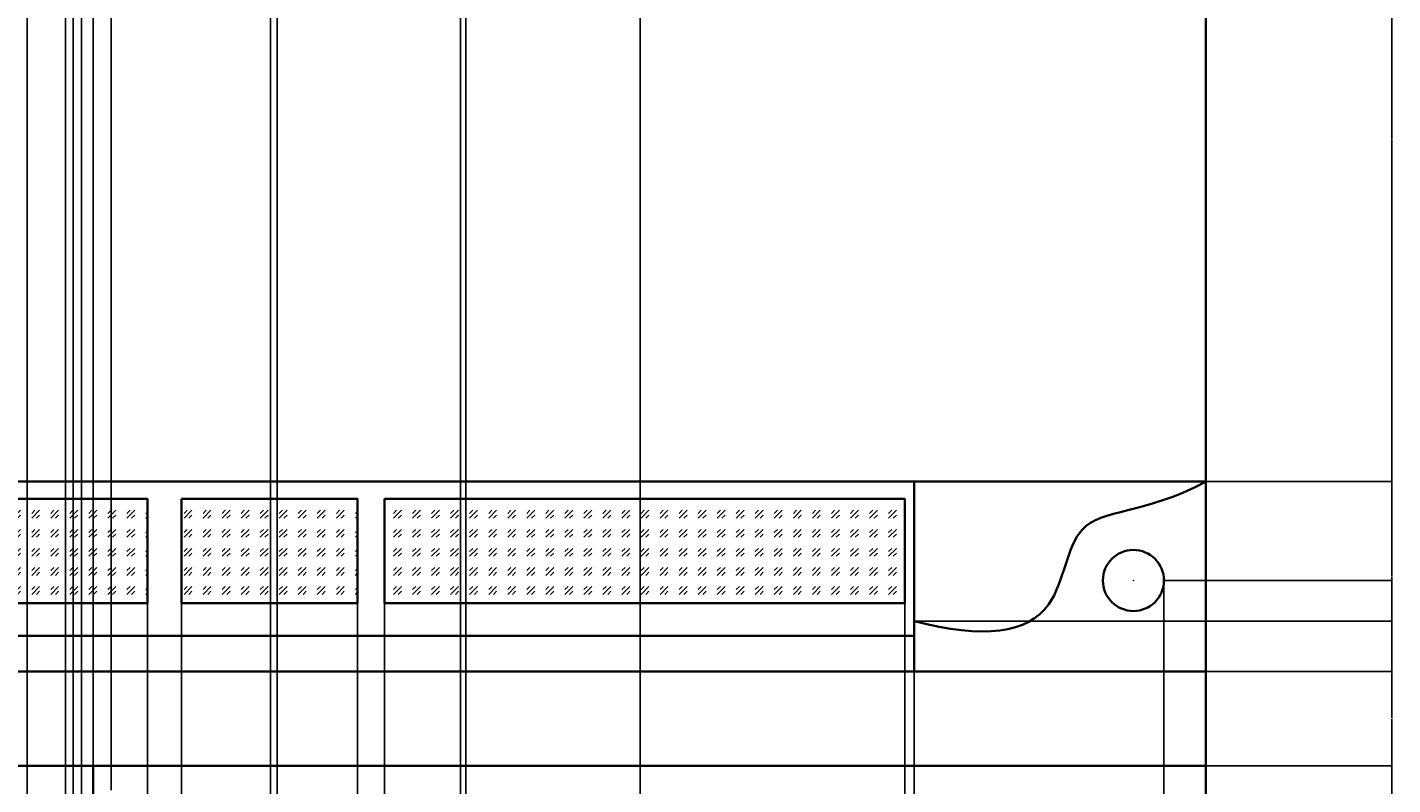
# Model space of a CAD drawing. Units: inches. Extents: x 1231 to 2151, y 481 to 2277.
# Tile 4 of 7: x 1542 to 2151, y 1035 to 1373. Entities that reach past the tile are written whole.
import ezdxf

# ---------------------------------------------------------------- set-up
doc = ezdxf.new("R2010")
doc.units = ezdxf.units.IN
doc.header["$MEASUREMENT"] = 0
for name, color, linetype, lineweight in [('A-ANNO-DIMS', 2, 'Continuous', 18), ('A-ELEV', 7, 'Continuous', 35), ('A-ELEV-PATT', 9, 'Continuous', 13)]:
    doc.layers.add(name, color=color, linetype=linetype, lineweight=lineweight)
doc.styles.get("Standard").update_dxf_attribs({"font": 'arial.ttf'})
doc.dimstyles.get("Standard").update_dxf_attribs({"dimtxt": 0.18, "dimasz": 0.18, "dimexe": 0.18, "dimexo": 0.0625, "dimgap": 0.09, "dimtad": 0, "dimtih": 1, "dimtoh": 1, "dimdec": 0, "dimzin": 0, "dimdsep": 46, "dimlunit": 3, "dimtxsty": 'Standard', "dimcen": 0.09, "dimadec": 0, "dimazin": 0, "dimtfac": 1, "dimtdec": 0, "dimtofl": 0, "dimtmove": 0, "dimatfit": 3, "dimfxl": 1, "dimtolj": 1, "dimtzin": 0, "dimarcsym": 0})

# ---------------------------------------------------------------- blocks, each defined once
blk = doc.blocks.new('*D4')
at = {"layer": 'A-ANNO-DIMS', "color": 0, "lineweight": -2, "transparency": 16777216}
for p, q in [((2067.75, 1043.69), (2150.62, 1043.69)), ((2150.44, 1043.51), (2150.44, 863.87)), ((2150.44, 683.87), (2150.44, 863.51)), ((2067.75, 683.69), (2150.62, 683.69))]:
    blk.add_line(p, q, dxfattribs=at)
at = {"layer": 'A-ANNO-DIMS', "color": 0, "transparency": 16777216}
for points in [[(2150.41, 1043.51), (2150.47, 1043.51), (2150.44, 1043.69)], [(2150.41, 683.87), (2150.47, 683.87), (2150.44, 683.69)]]:
    blk.add_solid(points, dxfattribs=at)
at = {"layer": 'Defpoints', "color": 0, "transparency": 16777216}
for p in [(2067.69, 1043.69), (2150.44, 1043.69), (2067.69, 683.69)]:
    blk.add_point(p, dxfattribs=at)
at = {"layer": 'A-ANNO-DIMS', "color": 0, "transparency": 16777216, "insert": (2150.44, 863.69), "char_height": 0.18, "attachment_point": 5}
blk.add_mtext('\\A1;360', dxfattribs=at)
blk = doc.blocks.new('*D5')
at = {"layer": 'A-ANNO-DIMS', "color": 0, "lineweight": -2, "transparency": 16777216}
for p, q in [((2067.75, 1085.71), (2150.62, 1085.71)), ((2150.44, 1085.53), (2150.44, 1064.88)), ((2150.44, 1043.87), (2150.44, 1064.52)), ((2067.75, 1043.69), (2150.62, 1043.69))]:
    blk.add_line(p, q, dxfattribs=at)
at = {"layer": 'A-ANNO-DIMS', "color": 0, "transparency": 16777216}
for points in [[(2150.41, 1085.53), (2150.47, 1085.53), (2150.44, 1085.71)], [(2150.41, 1043.87), (2150.47, 1043.87), (2150.44, 1043.69)]]:
    blk.add_solid(points, dxfattribs=at)
at = {"layer": 'Defpoints', "color": 0, "transparency": 16777216}
for p in [(2067.69, 1085.71), (2150.44, 1085.71), (2067.69, 1043.69)]:
    blk.add_point(p, dxfattribs=at)
at = {"layer": 'A-ANNO-DIMS', "color": 0, "transparency": 16777216, "insert": (2150.44, 1064.7), "char_height": 0.18, "attachment_point": 5}
blk.add_mtext('\\A1;42.02', dxfattribs=at)
blk = doc.blocks.new('*D6')
at = {"layer": 'A-ANNO-DIMS', "color": 0, "lineweight": -2, "transparency": 16777216}
for p, q in [((2067.75, 1170.34), (2150.62, 1170.34)), ((2150.44, 1170.16), (2150.44, 1128.2)), ((2150.44, 1085.89), (2150.44, 1127.84)), ((2067.75, 1085.71), (2150.62, 1085.71))]:
    blk.add_line(p, q, dxfattribs=at)
at = {"layer": 'A-ANNO-DIMS', "color": 0, "transparency": 16777216}
for points in [[(2150.41, 1170.16), (2150.47, 1170.16), (2150.44, 1170.34)], [(2150.41, 1085.89), (2150.47, 1085.89), (2150.44, 1085.71)]]:
    blk.add_solid(points, dxfattribs=at)
at = {"layer": 'Defpoints', "color": 0, "transparency": 16777216}
for p in [(2067.69, 1170.34), (2150.44, 1170.34), (2067.69, 1085.71)]:
    blk.add_point(p, dxfattribs=at)
at = {"layer": 'A-ANNO-DIMS', "color": 0, "transparency": 16777216, "insert": (2150.44, 1128.02), "char_height": 0.18, "attachment_point": 5}
blk.add_mtext('\\A1;84.63', dxfattribs=at)
blk = doc.blocks.new('*D7')
at = {"layer": 'A-ANNO-DIMS', "color": 0, "lineweight": -2, "transparency": 16777216}
for p, q in [((2067.75, 1475.54), (2150.62, 1475.54)), ((2150.44, 1475.36), (2150.44, 1323.12)), ((2150.44, 1170.52), (2150.44, 1322.76)), ((2067.75, 1170.34), (2150.62, 1170.34))]:
    blk.add_line(p, q, dxfattribs=at)
at = {"layer": 'A-ANNO-DIMS', "color": 0, "transparency": 16777216}
for points in [[(2150.41, 1475.36), (2150.47, 1475.36), (2150.44, 1475.54)], [(2150.41, 1170.52), (2150.47, 1170.52), (2150.44, 1170.34)]]:
    blk.add_solid(points, dxfattribs=at)
at = {"layer": 'Defpoints', "color": 0, "transparency": 16777216}
for p in [(2067.69, 1475.54), (2150.44, 1475.54), (2067.69, 1170.34)]:
    blk.add_point(p, dxfattribs=at)
at = {"layer": 'A-ANNO-DIMS', "color": 0, "transparency": 16777216, "insert": (2150.44, 1322.94), "char_height": 0.18, "attachment_point": 5}
blk.add_mtext('\\A1;305.2', dxfattribs=at)
blk = doc.blocks.new('*D34')
at = {"layer": 'A-ANNO-DIMS', "color": 0, "lineweight": -2, "transparency": 16777216}
for p, q in [((1489.86, 1037.75), (1489.86, 2276.71)), ((1490.04, 2276.53), (1515.72, 2276.53)), ((1542.2, 2276.53), (1516.51, 2276.53)), ((1542.38, 1043.75), (1542.38, 2276.71))]:
    blk.add_line(p, q, dxfattribs=at)
at = {"layer": 'A-ANNO-DIMS', "color": 0, "transparency": 16777216}
for points in [[(1490.04, 2276.56), (1490.04, 2276.5), (1489.86, 2276.53)], [(1542.2, 2276.56), (1542.2, 2276.5), (1542.38, 2276.53)]]:
    blk.add_solid(points, dxfattribs=at)
at = {"layer": 'Defpoints', "color": 0, "transparency": 16777216}
for p in [(1542.38, 2276.53), (1542.38, 1043.69), (1489.86, 1037.69)]:
    blk.add_point(p, dxfattribs=at)
at = {"layer": 'A-ANNO-DIMS', "color": 0, "transparency": 16777216, "insert": (1516.12, 2276.53), "char_height": 0.18, "attachment_point": 5}
blk.add_mtext('\\A1;52.52', dxfattribs=at)
blk = doc.blocks.new('*D35')
at = {"layer": 'A-ANNO-DIMS', "color": 0, "lineweight": -2, "transparency": 16777216}
for p, q in [((1542.38, 1043.75), (1542.38, 2276.71)), ((1542.56, 2276.53), (1556.6, 2276.53)), ((1571.58, 2276.53), (1557.53, 2276.53)), ((1571.76, 1043.75), (1571.76, 2276.71))]:
    blk.add_line(p, q, dxfattribs=at)
at = {"layer": 'A-ANNO-DIMS', "color": 0, "transparency": 16777216}
for points in [[(1542.56, 2276.56), (1542.56, 2276.5), (1542.38, 2276.53)], [(1571.58, 2276.56), (1571.58, 2276.5), (1571.76, 2276.53)]]:
    blk.add_solid(points, dxfattribs=at)
at = {"layer": 'Defpoints', "color": 0, "transparency": 16777216}
for p in [(1571.76, 2276.53), (1542.38, 1043.69), (1571.76, 1043.69)]:
    blk.add_point(p, dxfattribs=at)
at = {"layer": 'A-ANNO-DIMS', "color": 0, "transparency": 16777216, "insert": (1557.07, 2276.53), "char_height": 0.18, "attachment_point": 5}
blk.add_mtext('\\A1;29.385', dxfattribs=at)
blk = doc.blocks.new('*D36')
at = {"layer": 'A-ANNO-DIMS', "color": 0, "lineweight": -2, "transparency": 16777216}
for p, q in [((1571.76, 1043.75), (1571.76, 2276.71)), ((1571.94, 2276.53), (1575.38, 2276.53)), ((1579.61, 2276.53), (1576.17, 2276.53)), ((1579.79, 1032.87), (1579.79, 2276.71))]:
    blk.add_line(p, q, dxfattribs=at)
at = {"layer": 'A-ANNO-DIMS', "color": 0, "transparency": 16777216}
for points in [[(1571.94, 2276.56), (1571.94, 2276.5), (1571.76, 2276.53)], [(1579.61, 2276.56), (1579.61, 2276.5), (1579.79, 2276.53)]]:
    blk.add_solid(points, dxfattribs=at)
at = {"layer": 'Defpoints', "color": 0, "transparency": 16777216}
for p in [(1579.79, 2276.53), (1571.76, 1043.69), (1579.79, 1032.81)]:
    blk.add_point(p, dxfattribs=at)
at = {"layer": 'A-ANNO-DIMS', "color": 0, "transparency": 16777216, "insert": (1575.78, 2276.53), "char_height": 0.18, "attachment_point": 5}
blk.add_mtext('\\A1;8.033', dxfattribs=at)
blk = doc.blocks.new('*D50')
at = {"layer": 'A-ANNO-DIMS', "color": 0, "lineweight": -2, "transparency": 16777216}
for p, q in [((1542.38, 563.75), (1542.38, 2276.71)), ((1542.56, 2276.53), (1550.52, 2276.53)), ((1559.26, 2276.53), (1551.3, 2276.53)), ((1559.44, 576.65), (1559.44, 2276.71))]:
    blk.add_line(p, q, dxfattribs=at)
at = {"layer": 'A-ANNO-DIMS', "color": 0, "transparency": 16777216}
for points in [[(1542.56, 2276.56), (1542.56, 2276.5), (1542.38, 2276.53)], [(1559.26, 2276.56), (1559.26, 2276.5), (1559.44, 2276.53)]]:
    blk.add_solid(points, dxfattribs=at)
at = {"layer": 'Defpoints', "color": 0, "transparency": 16777216}
for p in [(1559.44, 2276.53), (1559.44, 576.59), (1542.38, 563.69)]:
    blk.add_point(p, dxfattribs=at)
at = {"layer": 'A-ANNO-DIMS', "color": 0, "transparency": 16777216, "insert": (1550.91, 2276.53), "char_height": 0.18, "attachment_point": 5}
blk.add_mtext('\\A1;17.07', dxfattribs=at)
blk = doc.blocks.new('*D69')
at = {"layer": 'A-ANNO-DIMS', "color": 0, "lineweight": -2, "transparency": 16777216}
for p, q in [((1512.01, 1085.65), (1512.01, 480.76)), ((1937.57, 1085.65), (1937.57, 480.76)), ((1512.19, 480.94), (1724.39, 480.94)), ((1937.39, 480.94), (1725.19, 480.94))]:
    blk.add_line(p, q, dxfattribs=at)
at = {"layer": 'A-ANNO-DIMS', "color": 0, "transparency": 16777216}
for points in [[(1512.19, 480.97), (1512.19, 480.91), (1512.01, 480.94)], [(1937.39, 480.97), (1937.39, 480.91), (1937.57, 480.94)]]:
    blk.add_solid(points, dxfattribs=at)
at = {"layer": 'Defpoints', "color": 0, "transparency": 16777216}
for p in [(1512.01, 1085.71), (1937.57, 1085.71), (1937.57, 480.94)]:
    blk.add_point(p, dxfattribs=at)
at = {"layer": 'A-ANNO-DIMS', "color": 0, "transparency": 16777216, "insert": (1724.79, 480.94), "char_height": 0.18, "attachment_point": 5}
blk.add_mtext('\\A1;425.6', dxfattribs=at)
blk = doc.blocks.new('*D71')
at = {"layer": 'A-ANNO-DIMS', "color": 0, "lineweight": -2, "transparency": 16777216}
for p, q in [((1517.5, 1116.1), (1517.5, 480.76)), ((1595.89, 1116.1), (1595.89, 480.76)), ((1517.68, 480.94), (1556.31, 480.94)), ((1595.71, 480.94), (1557.09, 480.94))]:
    blk.add_line(p, q, dxfattribs=at)
at = {"layer": 'A-ANNO-DIMS', "color": 0, "transparency": 16777216}
for points in [[(1517.68, 480.97), (1517.68, 480.91), (1517.5, 480.94)], [(1595.71, 480.97), (1595.71, 480.91), (1595.89, 480.94)]]:
    blk.add_solid(points, dxfattribs=at)
at = {"layer": 'Defpoints', "color": 0, "transparency": 16777216}
for p in [(1517.5, 1116.16), (1595.89, 1116.16), (1595.89, 480.94)]:
    blk.add_point(p, dxfattribs=at)
at = {"layer": 'A-ANNO-DIMS', "color": 0, "transparency": 16777216, "insert": (1556.7, 480.94), "char_height": 0.18, "attachment_point": 5}
blk.add_mtext('\\A1;78.39', dxfattribs=at)
blk = doc.blocks.new('*D72')
at = {"layer": 'A-ANNO-DIMS', "color": 0, "lineweight": -2, "transparency": 16777216}
for p, q in [((1595.89, 1116.1), (1595.89, 480.76)), ((1611.14, 1116.1), (1611.14, 480.76)), ((1596.07, 480.94), (1603.13, 480.94)), ((1610.96, 480.94), (1603.9, 480.94))]:
    blk.add_line(p, q, dxfattribs=at)
at = {"layer": 'A-ANNO-DIMS', "color": 0, "transparency": 16777216}
for points in [[(1596.07, 480.97), (1596.07, 480.91), (1595.89, 480.94)], [(1610.96, 480.97), (1610.96, 480.91), (1611.14, 480.94)]]:
    blk.add_solid(points, dxfattribs=at)
at = {"layer": 'Defpoints', "color": 0, "transparency": 16777216}
for p in [(1595.89, 1116.16), (1611.14, 1116.16), (1611.14, 480.94)]:
    blk.add_point(p, dxfattribs=at)
at = {"layer": 'A-ANNO-DIMS', "color": 0, "transparency": 16777216, "insert": (1603.52, 480.94), "char_height": 0.18, "attachment_point": 5}
blk.add_mtext('\\A1;15.25', dxfattribs=at)
blk = doc.blocks.new('*D73')
at = {"layer": 'A-ANNO-DIMS', "color": 0, "lineweight": -2, "transparency": 16777216}
for p, q in [((1611.14, 1116.1), (1611.14, 480.76)), ((1689.53, 1116.1), (1689.53, 480.76)), ((1611.32, 480.94), (1649.94, 480.94)), ((1689.35, 480.94), (1650.73, 480.94))]:
    blk.add_line(p, q, dxfattribs=at)
at = {"layer": 'A-ANNO-DIMS', "color": 0, "transparency": 16777216}
for points in [[(1611.32, 480.97), (1611.32, 480.91), (1611.14, 480.94)], [(1689.35, 480.97), (1689.35, 480.91), (1689.53, 480.94)]]:
    blk.add_solid(points, dxfattribs=at)
at = {"layer": 'Defpoints', "color": 0, "transparency": 16777216}
for p in [(1611.14, 1116.16), (1689.53, 1116.16), (1689.53, 480.94)]:
    blk.add_point(p, dxfattribs=at)
at = {"layer": 'A-ANNO-DIMS', "color": 0, "transparency": 16777216, "insert": (1650.34, 480.94), "char_height": 0.18, "attachment_point": 5}
blk.add_mtext('\\A1;78.39', dxfattribs=at)
blk = doc.blocks.new('*D74')
at = {"layer": 'A-ANNO-DIMS', "color": 0, "lineweight": -2, "transparency": 16777216}
for p, q in [((1689.53, 1116.1), (1689.53, 480.76)), ((1701.52, 1116.1), (1701.52, 480.76)), ((1689.71, 480.94), (1695.07, 480.94)), ((1701.34, 480.94), (1695.98, 480.94))]:
    blk.add_line(p, q, dxfattribs=at)
at = {"layer": 'A-ANNO-DIMS', "color": 0, "transparency": 16777216}
for points in [[(1689.71, 480.97), (1689.71, 480.91), (1689.53, 480.94)], [(1701.34, 480.97), (1701.34, 480.91), (1701.52, 480.94)]]:
    blk.add_solid(points, dxfattribs=at)
at = {"layer": 'Defpoints', "color": 0, "transparency": 16777216}
for p in [(1689.53, 1116.16), (1701.52, 1116.16), (1701.52, 480.94)]:
    blk.add_point(p, dxfattribs=at)
at = {"layer": 'A-ANNO-DIMS', "color": 0, "transparency": 16777216, "insert": (1695.53, 480.94), "char_height": 0.18, "attachment_point": 5}
blk.add_mtext('\\A1;11.992', dxfattribs=at)
blk = doc.blocks.new('*D75')
at = {"layer": 'A-ANNO-DIMS', "color": 0, "lineweight": -2, "transparency": 16777216}
for p, q in [((1701.52, 1116.1), (1701.52, 480.76)), ((1933.36, 1116.1), (1933.36, 480.76)), ((1701.7, 480.94), (1816.97, 480.94)), ((1933.18, 480.94), (1817.9, 480.94))]:
    blk.add_line(p, q, dxfattribs=at)
at = {"layer": 'A-ANNO-DIMS', "color": 0, "transparency": 16777216}
for points in [[(1701.7, 480.97), (1701.7, 480.91), (1701.52, 480.94)], [(1933.18, 480.97), (1933.18, 480.91), (1933.36, 480.94)]]:
    blk.add_solid(points, dxfattribs=at)
at = {"layer": 'Defpoints', "color": 0, "transparency": 16777216}
for p in [(1701.52, 1116.16), (1933.36, 1116.16), (1933.36, 480.94)]:
    blk.add_point(p, dxfattribs=at)
at = {"layer": 'A-ANNO-DIMS', "color": 0, "transparency": 16777216, "insert": (1817.44, 480.94), "char_height": 0.18, "attachment_point": 5}
blk.add_mtext('\\A1;231.83', dxfattribs=at)
blk = doc.blocks.new('*D80')
at = {"layer": 'A-ANNO-DIMS', "color": 0, "lineweight": -2, "transparency": 16777216}
for p, q in [((1937.57, 1170.27), (1937.57, 480.76)), ((2048.89, 1126.2), (2048.89, 480.76)), ((1937.75, 480.94), (1992.79, 480.94)), ((2048.71, 480.94), (1993.67, 480.94))]:
    blk.add_line(p, q, dxfattribs=at)
at = {"layer": 'A-ANNO-DIMS', "color": 0, "transparency": 16777216}
for points in [[(1937.75, 480.97), (1937.75, 480.91), (1937.57, 480.94)], [(2048.71, 480.97), (2048.71, 480.91), (2048.89, 480.94)]]:
    blk.add_solid(points, dxfattribs=at)
at = {"layer": 'Defpoints', "color": 0, "transparency": 16777216}
for p in [(1937.57, 1170.34), (2048.89, 1126.26), (2048.89, 480.94)]:
    blk.add_point(p, dxfattribs=at)
at = {"layer": 'A-ANNO-DIMS', "color": 0, "transparency": 16777216, "insert": (1993.23, 480.94), "char_height": 0.18, "attachment_point": 5}
blk.add_mtext('\\A1;111.31', dxfattribs=at)
blk = doc.blocks.new('*D81')
at = {"layer": 'A-ANNO-DIMS', "color": 0, "lineweight": -2, "transparency": 16777216}
for p, q in [((2048.95, 1126.26), (2150.62, 1126.26)), ((2150.44, 1126.08), (2150.44, 1106.17)), ((2150.44, 1085.89), (2150.44, 1105.8)), ((1937.63, 1085.71), (2150.62, 1085.71))]:
    blk.add_line(p, q, dxfattribs=at)
at = {"layer": 'A-ANNO-DIMS', "color": 0, "transparency": 16777216}
for points in [[(2150.41, 1126.08), (2150.47, 1126.08), (2150.44, 1126.26)], [(2150.41, 1085.89), (2150.47, 1085.89), (2150.44, 1085.71)]]:
    blk.add_solid(points, dxfattribs=at)
at = {"layer": 'Defpoints', "color": 0, "transparency": 16777216}
for p in [(2048.89, 1126.26), (2150.44, 1126.26), (1937.57, 1085.71)]:
    blk.add_point(p, dxfattribs=at)
at = {"layer": 'A-ANNO-DIMS', "color": 0, "transparency": 16777216, "insert": (2150.44, 1105.98), "char_height": 0.18, "attachment_point": 5}
blk.add_mtext('\\A1;40.55', dxfattribs=at)
blk = doc.blocks.new('*D82')
at = {"layer": 'A-ANNO-DIMS', "color": 0, "lineweight": -2, "transparency": 16777216}
for p, q in [((1937.63, 1108.18), (2150.62, 1108.18)), ((2150.44, 1108), (2150.44, 1097.13)), ((2150.44, 1085.89), (2150.44, 1096.76)), ((1937.63, 1085.71), (2150.62, 1085.71))]:
    blk.add_line(p, q, dxfattribs=at)
at = {"layer": 'A-ANNO-DIMS', "color": 0, "transparency": 16777216}
for points in [[(2150.41, 1108), (2150.47, 1108), (2150.44, 1108.18)], [(2150.41, 1085.89), (2150.47, 1085.89), (2150.44, 1085.71)]]:
    blk.add_solid(points, dxfattribs=at)
at = {"layer": 'Defpoints', "color": 0, "transparency": 16777216}
for p in [(1937.57, 1108.18), (2150.44, 1108.18), (1937.57, 1085.71)]:
    blk.add_point(p, dxfattribs=at)
at = {"layer": 'A-ANNO-DIMS', "color": 0, "transparency": 16777216, "insert": (2150.44, 1096.94), "char_height": 0.18, "attachment_point": 5}
blk.add_mtext('\\A1;22.473', dxfattribs=at)
blk = doc.blocks.new('*D90')
at = {"layer": 'A-ANNO-DIMS', "color": 0, "lineweight": -2, "transparency": 16777216}
for p, q in [((1566.56, 1479.25), (1566.56, 480.76)), ((1562.79, 1475.48), (1562.79, 480.76)), ((1562.97, 480.94), (1564.3, 480.94)), ((1566.38, 480.94), (1565.05, 480.94))]:
    blk.add_line(p, q, dxfattribs=at)
at = {"layer": 'A-ANNO-DIMS', "color": 0, "transparency": 16777216}
for points in [[(1562.97, 480.97), (1562.97, 480.91), (1562.79, 480.94)], [(1566.38, 480.97), (1566.38, 480.91), (1566.56, 480.94)]]:
    blk.add_solid(points, dxfattribs=at)
at = {"layer": 'Defpoints', "color": 0, "transparency": 16777216}
for p in [(1566.56, 1479.32), (1562.79, 1475.54), (1566.56, 480.94)]:
    blk.add_point(p, dxfattribs=at)
at = {"layer": 'A-ANNO-DIMS', "color": 0, "transparency": 16777216, "insert": (1564.68, 480.94), "char_height": 0.18, "attachment_point": 5}
blk.add_mtext('\\A1;3.771', dxfattribs=at)
blk = doc.blocks.new('*D91')
at = {"layer": 'A-ANNO-DIMS', "color": 0, "lineweight": -2, "transparency": 16777216}
for p, q in [((1566.56, 1479.25), (1566.56, 480.76)), ((1650.77, 1479.25), (1650.77, 480.76)), ((1566.74, 480.94), (1608.34, 480.94)), ((1650.59, 480.94), (1608.99, 480.94))]:
    blk.add_line(p, q, dxfattribs=at)
at = {"layer": 'A-ANNO-DIMS', "color": 0, "transparency": 16777216}
for points in [[(1566.74, 480.97), (1566.74, 480.91), (1566.56, 480.94)], [(1650.59, 480.97), (1650.59, 480.91), (1650.77, 480.94)]]:
    blk.add_solid(points, dxfattribs=at)
at = {"layer": 'Defpoints', "color": 0, "transparency": 16777216}
for p in [(1566.56, 1479.32), (1650.77, 1479.32), (1650.77, 480.94)]:
    blk.add_point(p, dxfattribs=at)
at = {"layer": 'A-ANNO-DIMS', "color": 0, "transparency": 16777216, "insert": (1608.66, 480.94), "char_height": 0.18, "attachment_point": 5}
blk.add_mtext('\\A1;84.2', dxfattribs=at)
blk = doc.blocks.new('*D92')
at = {"layer": 'A-ANNO-DIMS', "color": 0, "lineweight": -2, "transparency": 16777216}
for p, q in [((1653.67, 1479.25), (1653.67, 480.76)), ((1735.42, 1479.25), (1735.42, 480.76)), ((1653.85, 480.94), (1694.15, 480.94)), ((1735.24, 480.94), (1694.94, 480.94))]:
    blk.add_line(p, q, dxfattribs=at)
at = {"layer": 'A-ANNO-DIMS', "color": 0, "transparency": 16777216}
for points in [[(1653.85, 480.97), (1653.85, 480.91), (1653.67, 480.94)], [(1735.24, 480.97), (1735.24, 480.91), (1735.42, 480.94)]]:
    blk.add_solid(points, dxfattribs=at)
at = {"layer": 'Defpoints', "color": 0, "transparency": 16777216}
for p in [(1653.67, 1479.32), (1735.42, 1479.32), (1735.42, 480.94)]:
    blk.add_point(p, dxfattribs=at)
at = {"layer": 'A-ANNO-DIMS', "color": 0, "transparency": 16777216, "insert": (1694.55, 480.94), "char_height": 0.18, "attachment_point": 5}
blk.add_mtext('\\A1;81.75', dxfattribs=at)
blk = doc.blocks.new('*D93')
at = {"layer": 'A-ANNO-DIMS', "color": 0, "lineweight": -2, "transparency": 16777216}
for p, q in [((1737.75, 1479.25), (1737.75, 480.76)), ((1815.54, 1479.25), (1815.54, 480.76)), ((1737.93, 480.94), (1776.25, 480.94)), ((1815.36, 480.94), (1777.04, 480.94))]:
    blk.add_line(p, q, dxfattribs=at)
at = {"layer": 'A-ANNO-DIMS', "color": 0, "transparency": 16777216}
for points in [[(1737.93, 480.97), (1737.93, 480.91), (1737.75, 480.94)], [(1815.36, 480.97), (1815.36, 480.91), (1815.54, 480.94)]]:
    blk.add_solid(points, dxfattribs=at)
at = {"layer": 'Defpoints', "color": 0, "transparency": 16777216}
for p in [(1737.75, 1479.32), (1815.54, 1479.32), (1815.54, 480.94)]:
    blk.add_point(p, dxfattribs=at)
at = {"layer": 'A-ANNO-DIMS', "color": 0, "transparency": 16777216, "insert": (1776.64, 480.94), "char_height": 0.18, "attachment_point": 5}
blk.add_mtext('\\A1;77.79', dxfattribs=at)
blk = doc.blocks.new('*D97')
at = {"layer": 'A-ANNO-DIMS', "color": 0, "lineweight": -2, "transparency": 16777216}
for p, q in [((2035.19, 1126.26), (2035.37, 1126.26)), ((2035.28, 1126.17), (2035.28, 1126.35)), ((2057.05, 1126.32), (2049.07, 1126.3))]:
    blk.add_line(p, q, dxfattribs=at)
at = {"layer": 'A-ANNO-DIMS', "color": 0, "transparency": 16777216}
blk.add_solid([(2049.07, 1126.33), (2049.07, 1126.27), (2048.89, 1126.3)], dxfattribs=at)
at = {"layer": 'Defpoints', "color": 0, "transparency": 16777216}
for p in [(2021.67, 1126.22), (2048.89, 1126.3)]:
    blk.add_point(p, dxfattribs=at)
at = {"layer": 'A-ANNO-DIMS', "color": 0, "transparency": 16777216, "insert": (2057.54, 1126.32), "char_height": 0.18, "attachment_point": 5}
blk.add_mtext('\\A1;∅27.22', dxfattribs=at)

msp = doc.modelspace()

# ---------------------------------------------------------------- hatches: boundary and pattern name
at = {"layer": 'A-ELEV-PATT'}
h = msp.add_hatch(dxfattribs=at)
h.set_pattern_fill('GOST_GLASS', color=256)
h.set_pattern_definition([(45, (0, 0), (8.485281, 0), [5, -7]), (45, (2.1213, 0), (8.485281, 0), [2, -10]), (45, (0, 2.1213), (8.485281, 0), [2, -10])])
h.paths.add_polyline_path([(1595.8928, 1116.1584), (1595.8928, 1162.5965), (1517.5039, 1162.5965), (1517.5039, 1116.1584)])
h.paths.add_polyline_path([(1689.5303, 1162.5965), (1611.1414, 1162.5965), (1611.1414, 1116.1584), (1689.5303, 1116.1584)])
h.paths.add_polyline_path([(1933.3556, 1116.1584), (1933.3556, 1162.5965), (1701.522, 1162.5965), (1701.522, 1116.1584)])

# ---------------------------------------------------------------- linework, layer by layer
at = {"layer": 'A-ELEV'}
for p, q in [((2067.4747, 563.6912), (2067.4747, 2193.7789)), ((1314.2408, 1170.3351), (2067.6855, 1170.3351)), ((1937.5725, 1170.3351), (1937.5725, 1085.7079)), ((1512.0105, 1101.5825), (1937.5725, 1101.5825)), ((1314.2408, 1085.7079), (2067.6855, 1085.7079)), ((1314.2408, 1043.6912), (2067.6855, 1043.6912)), ((1571.76, 1043.6912), (1571.76, 683.6912))]:
    msp.add_line(p, q, dxfattribs=at)
for points in [[(1517.5039, 1162.5965), (1595.8928, 1162.5965), (1595.8928, 1116.1584), (1517.5039, 1116.1584)], [(1611.1414, 1162.5965), (1689.5303, 1162.5965), (1689.5303, 1116.1584), (1611.1414, 1116.1584)], [(1701.522, 1162.5965), (1933.3556, 1162.5965), (1933.3556, 1116.1584), (1701.522, 1116.1584)]]:
    msp.add_lwpolyline(points, close=True, dxfattribs=at)
msp.add_circle((2035.2782, 1126.2615), 13.6087, dxfattribs=at)
msp.add_open_spline([(1937.5725, 1108.1804), (1968.4724, 1100.1431), (2003.0162, 1104.2254), (2006.7806, 1161.1291), (2039.5193, 1155.3279), (2067.6855, 1170.3351)], degree=3, knots=[0, 0, 0, 0, 67.81601683, 117.98522858, 181.42476167, 181.42476167, 181.42476167, 181.42476167], dxfattribs=at)

# ---------------------------------------------------------------- dimensions: what is measured, and where the dimension line sits
at = {"layer": 'A-ANNO-DIMS'}
for base, p1, p2, override, picture, middle in [((1542.3752, 2276.5289), (1489.8565, 1037.6872), (1542.3752, 1043.6912), {"dimdec": 2, "dimlfac": 1, "dimrnd": 0, "dimzin": 0, "dimdsep": 46, "dimlunit": 2}, '*D34', (1516.1158, 2276.5289)), ((1571.76, 2276.5289), (1542.3752, 1043.6912), (1571.76, 1043.6912), {"dimdec": 3, "dimlfac": 1, "dimrnd": 0, "dimzin": 0, "dimdsep": 46, "dimlunit": 2}, '*D35', (1557.0676, 2276.5289)), ((1559.4446, 2276.5289), (1542.3752, 563.6912), (1559.4446, 576.5889), {"dimdec": 2, "dimlfac": 1, "dimrnd": 0, "dimzin": 0, "dimdsep": 46, "dimlunit": 2}, '*D50', (1550.9099, 2276.5289)), ((1579.7928, 2276.5289), (1571.76, 1043.6912), (1579.7928, 1032.8111), {"dimdec": 3, "dimlfac": 1, "dimrnd": 0, "dimzin": 0, "dimdsep": 46, "dimlunit": 2}, '*D36', (1575.7764, 2276.5289)), ((1566.5626, 480.9412), (1562.7916, 1475.5441), (1566.5626, 1479.3152), {"dimdec": 3, "dimlfac": 1, "dimrnd": 0, "dimzin": 0, "dimdsep": 46, "dimlunit": 2}, '*D90', (1564.6771, 480.9412)), ((1650.766, 480.9412), (1566.5626, 1479.3152), (1650.766, 1479.3152), {"dimdec": 1, "dimlfac": 1, "dimrnd": 0, "dimzin": 0, "dimdsep": 46, "dimlunit": 2}, '*D91', (1608.6643, 480.9412)), ((1735.4237, 480.9412), (1653.6719, 1479.3152), (1735.4237, 1479.3152), {"dimdec": 2, "dimlfac": 1, "dimrnd": 0, "dimzin": 0, "dimdsep": 46, "dimlunit": 2}, '*D92', (1694.5478, 480.9412)), ((1815.5376, 480.9412), (1737.7463, 1479.3152), (1815.5376, 1479.3152), {"dimdec": 2, "dimlfac": 1, "dimrnd": 0, "dimzin": 0, "dimdsep": 46, "dimlunit": 2}, '*D93', (1776.642, 480.9412)), ((2048.8868, 480.9412), (1937.5725, 1170.3351), (2048.8868, 1126.2615), {"dimdec": 2, "dimlfac": 1, "dimrnd": 0, "dimzin": 0, "dimdsep": 46, "dimlunit": 2}, '*D80', (1993.2297, 480.9412)), ((1595.8928, 480.9412), (1517.5039, 1116.1584), (1595.8928, 1116.1584), {"dimdec": 2, "dimlfac": 1, "dimrnd": 0, "dimzin": 0, "dimdsep": 46, "dimlunit": 2}, '*D71', (1556.6984, 480.9412)), ((1611.1414, 480.9412), (1595.8928, 1116.1584), (1611.1414, 1116.1584), {"dimdec": 2, "dimlfac": 1, "dimrnd": 0, "dimzin": 0, "dimdsep": 46, "dimlunit": 2}, '*D72', (1603.5171, 480.9412)), ((1689.5303, 480.9412), (1611.1414, 1116.1584), (1689.5303, 1116.1584), {"dimdec": 2, "dimlfac": 1, "dimrnd": 0, "dimzin": 0, "dimdsep": 46, "dimlunit": 2}, '*D73', (1650.3359, 480.9412)), ((1701.522, 480.9412), (1689.5303, 1116.1584), (1701.522, 1116.1584), {"dimdec": 3, "dimlfac": 1, "dimrnd": 0, "dimzin": 0, "dimdsep": 46, "dimlunit": 2}, '*D74', (1695.5261, 480.9412)), ((1933.3556, 480.9412), (1701.522, 1116.1584), (1933.3556, 1116.1584), {"dimdec": 2, "dimlfac": 1, "dimrnd": 0, "dimzin": 0, "dimdsep": 46, "dimlunit": 2}, '*D75', (1817.4388, 480.9412)), ((1937.5725, 480.9412), (1512.0105, 1085.7079), (1937.5725, 1085.7079), {"dimdec": 1, "dimlfac": 1, "dimrnd": 0, "dimzin": 0, "dimdsep": 46, "dimlunit": 2}, '*D69', (1724.7915, 480.9412))]:
    dim = msp.add_linear_dim(base=base, p1=p1, p2=p2, dimstyle='Standard', override=override, dxfattribs=at)
    dim.commit()
    dim.dimension.update_dxf_attribs({"geometry": picture, "text_midpoint": middle})
for base, p1, p2, override, picture, middle in [((2150.4355, 1475.5441), (2067.6855, 1170.3351), (2067.6855, 1475.5441), {"dimdec": 1, "dimlfac": 1, "dimrnd": 0, "dimzin": 0, "dimdsep": 46, "dimlunit": 2}, '*D7', (2150.4355, 1322.9396)), ((2150.4355, 1170.3351), (2067.6855, 1085.7079), (2067.6855, 1170.3351), {"dimdec": 2, "dimlfac": 1, "dimrnd": 0, "dimzin": 0, "dimdsep": 46, "dimlunit": 2}, '*D6', (2150.4355, 1128.0215)), ((2150.4355, 1126.2615), (1937.5725, 1085.7079), (2048.8868, 1126.2615), {"dimdec": 2, "dimlfac": 1, "dimrnd": 0, "dimzin": 0, "dimdsep": 46, "dimlunit": 2}, '*D81', (2150.4355, 1105.9847)), ((2150.43552, 1108.18041), (1937.57246, 1085.70788), (1937.57246, 1108.18041), {"dimdec": 3, "dimlfac": 1, "dimrnd": 0, "dimzin": 0, "dimdsep": 46, "dimlunit": 2}, '*D82', (2150.43552, 1096.94414)), ((2150.4355, 1085.7079), (2067.6855, 1043.6912), (2067.6855, 1085.7079), {"dimdec": 2, "dimlfac": 1, "dimrnd": 0, "dimzin": 0, "dimdsep": 46, "dimlunit": 2}, '*D5', (2150.4355, 1064.6996)), ((2150.4355, 1043.6912), (2067.6855, 683.6912), (2067.6855, 1043.6912), {"dimdec": 0, "dimlfac": 1, "dimrnd": 0, "dimzin": 0, "dimdsep": 46, "dimlunit": 2}, '*D4', (2150.4355, 863.6912))]:
    dim = msp.add_linear_dim(base=base, p1=p1, p2=p2, angle=90, dimstyle='Standard', override=override, dxfattribs=at)
    dim.commit()
    dim.dimension.update_dxf_attribs({"geometry": picture, "text_midpoint": middle})
dim = msp.add_diameter_dim_2p(p1=(2021.6696, 1126.223), p2=(2048.8868, 1126.3), dimstyle='Standard', override={"dimdec": 2, "dimlfac": 1, "dimrnd": 0, "dimzin": 0, "dimdsep": 46, "dimlunit": 2}, dxfattribs=at)
dim.commit()
dim.dimension.update_dxf_attribs({"geometry": '*D97', "text_midpoint": (2057.0519, 1126.323), "dimtype": 163})

doc.saveas('drawing.dxf')
